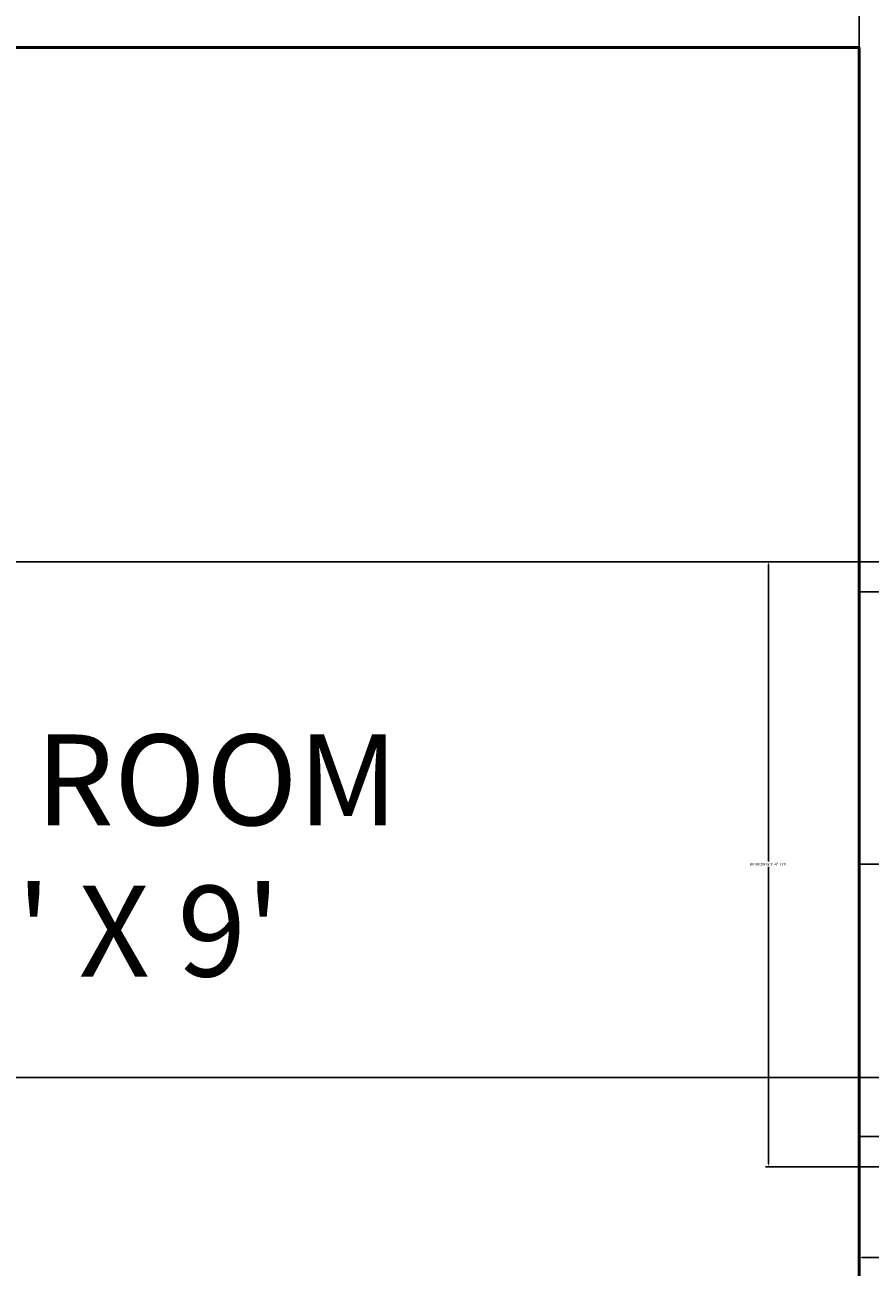
# Model space of a CAD drawing. Units: inches. Extents: x 37 to 824, y -700 to 234.
# Tile 65 of 77: x 364 to 420, y -75 to 8. Entities that reach past the tile are written whole.
import ezdxf

# ---------------------------------------------------------------- set-up
doc = ezdxf.new("R2010")
doc.units = ezdxf.units.IN
doc.header["$MEASUREMENT"] = 0
for name, color, linetype, lineweight in [('A-ANNO-DIMS', 2, 'Continuous', 18), ('A-AREA-IDEN', 3, 'Continuous', 18), ('A-GLAZ', 4, 'Continuous', 25), ('A-WALL', 2, 'Continuous', 50)]:
    doc.layers.add(name, color=color, linetype=linetype, lineweight=lineweight)
doc.styles.get("Standard").update_dxf_attribs({"font": 'arial.ttf'})
doc.dimstyles.get("Standard").update_dxf_attribs({"dimtxt": 0.18, "dimasz": 0.18, "dimexe": 0.18, "dimexo": 0.0625, "dimgap": 0.09, "dimtad": 0, "dimtih": 1, "dimtoh": 1, "dimdec": 1, "dimzin": 0, "dimdsep": 46, "dimlunit": 4, "dimtxsty": 'Standard', "dimcen": 0.09, "dimadec": 0, "dimazin": 0, "dimtfac": 1, "dimtdec": 1, "dimtofl": 0, "dimtmove": 0, "dimatfit": 3, "dimfxl": 1, "dimtolj": 1, "dimtzin": 0, "dimarcsym": 0})

# ---------------------------------------------------------------- blocks, each defined once
blk = doc.blocks.new('WIN-900')
for p, q in [((0, 9), (0, 0)), ((2, 9), (2, 0)), ((20, 9), (20, 0)), ((38, 9), (38, 0)), ((40, 9), (40, 0)), ((38, 5.5), (2, 5.5)), ((38, 3.5), (2, 3.5))]:
    blk.add_line(p, q)
blk = doc.blocks.new('*D38')
at = {"layer": 'A-ANNO-DIMS', "color": 0, "lineweight": -2, "ltscale": 0.5, "transparency": 16777216}
for p, q in [((419.015, -27.91), (412.897, -27.91)), ((413.077, -28.09), (413.077, -47.726)), ((413.077, -67.73), (413.077, -48.093)), ((419.015, -67.91), (412.897, -67.91))]:
    blk.add_line(p, q, dxfattribs=at)
at = {"layer": 'A-ANNO-DIMS', "color": 0, "ltscale": 0.5, "transparency": 16777216}
for points in [[(413.047, -28.09), (413.107, -28.09), (413.077, -27.91)], [(413.047, -67.73), (413.107, -67.73), (413.077, -67.91)]]:
    blk.add_solid(points, dxfattribs=at)
at = {"layer": 'Defpoints', "color": 0, "ltscale": 0.5, "transparency": 16777216}
for p in [(419.077, -27.91), (413.077, -67.91), (419.077, -67.91)]:
    blk.add_point(p, dxfattribs=at)
at = {"layer": 'A-ANNO-DIMS', "color": 0, "ltscale": 0.5, "transparency": 16777216, "insert": (413.077, -47.91), "char_height": 0.18, "attachment_point": 5}
blk.add_mtext('\\A1;WINDOW W 3\'-4" TYP.', dxfattribs=at)
blk = doc.blocks.new('*D39')
at = {"layer": 'A-ANNO-DIMS', "color": 0, "lineweight": -2, "ltscale": 0.5, "transparency": 16777216}
for p, q in [((419.077, -67.972), (419.077, -74.09)), ((428.077, -67.972), (428.077, -74.09)), ((419.257, -73.91), (422.939, -73.91)), ((427.897, -73.91), (424.216, -73.91))]:
    blk.add_line(p, q, dxfattribs=at)
at = {"layer": 'A-ANNO-DIMS', "color": 0, "ltscale": 0.5, "transparency": 16777216}
for points in [[(419.257, -73.88), (419.257, -73.94), (419.077, -73.91)], [(427.897, -73.88), (427.897, -73.94), (428.077, -73.91)]]:
    blk.add_solid(points, dxfattribs=at)
at = {"layer": 'Defpoints', "color": 0, "ltscale": 0.5, "transparency": 16777216}
for p in [(419.077, -67.91), (428.077, -67.91), (428.077, -73.91)]:
    blk.add_point(p, dxfattribs=at)
at = {"layer": 'A-ANNO-DIMS', "color": 0, "ltscale": 0.5, "transparency": 16777216, "insert": (423.577, -73.91), "char_height": 0.18, "attachment_point": 5}
blk.add_mtext('\\A1;0\'-9" TYP.', dxfattribs=at)
blk = doc.blocks.new('*D62')
at = {"layer": 'A-ANNO-DIMS', "color": 0, "lineweight": -2, "ltscale": 0.5, "transparency": 16777216}
for p, q in [((419.015, 6.09), (78.159, 6.09)), ((78.339, 5.91), (78.339, -10.728)), ((78.339, -27.73), (78.339, -11.091)), ((419.015, -27.91), (78.159, -27.91))]:
    blk.add_line(p, q, dxfattribs=at)
at = {"layer": 'A-ANNO-DIMS', "color": 0, "ltscale": 0.5, "transparency": 16777216}
for points in [[(78.309, 5.91), (78.369, 5.91), (78.339, 6.09)], [(78.309, -27.73), (78.369, -27.73), (78.339, -27.91)]]:
    blk.add_solid(points, dxfattribs=at)
at = {"layer": 'Defpoints', "color": 0, "ltscale": 0.5, "transparency": 16777216}
for p in [(419.077, 6.09), (78.339, -27.91), (419.077, -27.91)]:
    blk.add_point(p, dxfattribs=at)
at = {"layer": 'A-ANNO-DIMS', "color": 0, "ltscale": 0.5, "transparency": 16777216, "insert": (78.339, -10.91), "char_height": 0.18, "attachment_point": 5}
blk.add_mtext('\\A1;2\'-10"', dxfattribs=at)
blk = doc.blocks.new('*D79')
at = {"layer": 'A-ANNO-DIMS', "color": 0, "lineweight": -2, "ltscale": 0.5, "transparency": 16777216}
for p, q in [((299.14, -62.022), (513.773, -62.022)), ((513.593, -62.202), (513.593, -81.784)), ((513.593, -101.73), (513.593, -82.148)), ((296.14, -101.91), (513.773, -101.91))]:
    blk.add_line(p, q, dxfattribs=at)
at = {"layer": 'A-ANNO-DIMS', "color": 0, "ltscale": 0.5, "transparency": 16777216}
for points in [[(513.563, -62.202), (513.623, -62.202), (513.593, -62.022)], [(513.563, -101.73), (513.623, -101.73), (513.593, -101.91)]]:
    blk.add_solid(points, dxfattribs=at)
at = {"layer": 'Defpoints', "color": 0, "ltscale": 0.5, "transparency": 16777216}
for p in [(299.077, -62.022), (296.077, -101.91), (513.593, -101.91)]:
    blk.add_point(p, dxfattribs=at)
at = {"layer": 'A-ANNO-DIMS', "color": 0, "ltscale": 0.5, "transparency": 16777216, "insert": (513.593, -81.966), "char_height": 0.18, "attachment_point": 5}
blk.add_mtext('\\A1;3\'-4"', dxfattribs=at)
blk = doc.blocks.new('*D83')
at = {"layer": 'A-ANNO-DIMS', "color": 0, "lineweight": -2, "ltscale": 0.5, "transparency": 16777216}
for p, q in [((358.132, -206.847), (358.132, 234.17)), ((419.077, -206.847), (419.077, 234.17)), ((358.312, 233.99), (388.275, 233.99)), ((418.897, 233.99), (388.934, 233.99))]:
    blk.add_line(p, q, dxfattribs=at)
at = {"layer": 'A-ANNO-DIMS', "color": 0, "ltscale": 0.5, "transparency": 16777216}
for points in [[(358.312, 234.02), (358.312, 233.96), (358.132, 233.99)], [(418.897, 234.02), (418.897, 233.96), (419.077, 233.99)]]:
    blk.add_solid(points, dxfattribs=at)
at = {"layer": 'Defpoints', "color": 0, "ltscale": 0.5, "transparency": 16777216}
for p in [(419.077, 233.99), (358.132, -206.91), (419.077, -206.91)]:
    blk.add_point(p, dxfattribs=at)
at = {"layer": 'A-ANNO-DIMS', "color": 0, "ltscale": 0.5, "transparency": 16777216, "insert": (388.605, 233.99), "char_height": 0.18, "attachment_point": 5}
blk.add_mtext('\\A1;5\'-1"', dxfattribs=at)

msp = doc.modelspace()

# ---------------------------------------------------------------- linework, layer by layer
at = {"layer": 'A-WALL'}
for q in [(299.077, 6.09), (419.077, -101.91)]:
    msp.add_line((419.077, 6.09), q, dxfattribs=at)

# ---------------------------------------------------------------- block references
at = {"layer": 'A-GLAZ', "rotation": 270.0000000000001}
msp.add_blockref('WIN-900', (419.077, -27.909), dxfattribs=at)

# ---------------------------------------------------------------- texts
at = {"layer": 'A-AREA-IDEN', "insert": (346.954, -39.332), "char_height": 6, "attachment_point": 1}
msp.add_mtext_dynamic_manual_height_columns("BED ROOM\\P    10' X 9'", width=88.32168, gutter_width=1, heights=[0], dxfattribs=at)

# ---------------------------------------------------------------- dimensions: what is measured, and where the dimension line sits
at = {"layer": 'A-ANNO-DIMS', "ltscale": 0.5}
dim = msp.add_linear_dim(base=(419.077, 233.99), p1=(358.132, -206.91), p2=(419.077, -206.91), dimstyle='Standard', override={"dimdec": 1, "dimlfac": 1, "dimrnd": 0, "dimzin": 1, "dimdsep": 46, "dimlunit": 4, "dimfrac": 2}, dxfattribs=at)
dim.commit()
dim.dimension.update_dxf_attribs({"geometry": '*D83', "text_midpoint": (388.605, 233.99)})
for base, p1, p2, picture, middle in [((78.339, -27.91), (419.077, 6.09), (419.077, -27.91), '*D62', (78.339, -10.91)), ((513.593, -101.91), (299.077, -62.022), (296.077, -101.91), '*D79', (513.593, -81.966))]:
    dim = msp.add_linear_dim(base=base, p1=p1, p2=p2, angle=90, dimstyle='Standard', override={"dimdec": 1, "dimlfac": 1, "dimrnd": 0, "dimzin": 1, "dimdsep": 46, "dimlunit": 4, "dimfrac": 2}, dxfattribs=at)
    dim.commit()
    dim.dimension.update_dxf_attribs({"geometry": picture, "text_midpoint": middle})
for base, p1, p2, angle, text, picture, middle in [((413.077, -67.91), (419.077, -27.91), (419.077, -67.91), 270, 'WINDOW W <> TYP.', '*D38', (413.077, -47.91)), ((428.077, -73.91), (419.077, -67.91), (428.077, -67.91), 0, '<> TYP.', '*D39', (423.577, -73.91))]:
    dim = msp.add_linear_dim(base=base, p1=p1, p2=p2, angle=angle, text=text, dimstyle='Standard', override={"dimdec": 1, "dimlfac": 1, "dimrnd": 0, "dimzin": 1, "dimdsep": 46, "dimlunit": 4, "dimfrac": 2}, dxfattribs=at)
    dim.commit()
    dim.dimension.update_dxf_attribs({"geometry": picture, "text_midpoint": middle})

doc.saveas('drawing.dxf')
